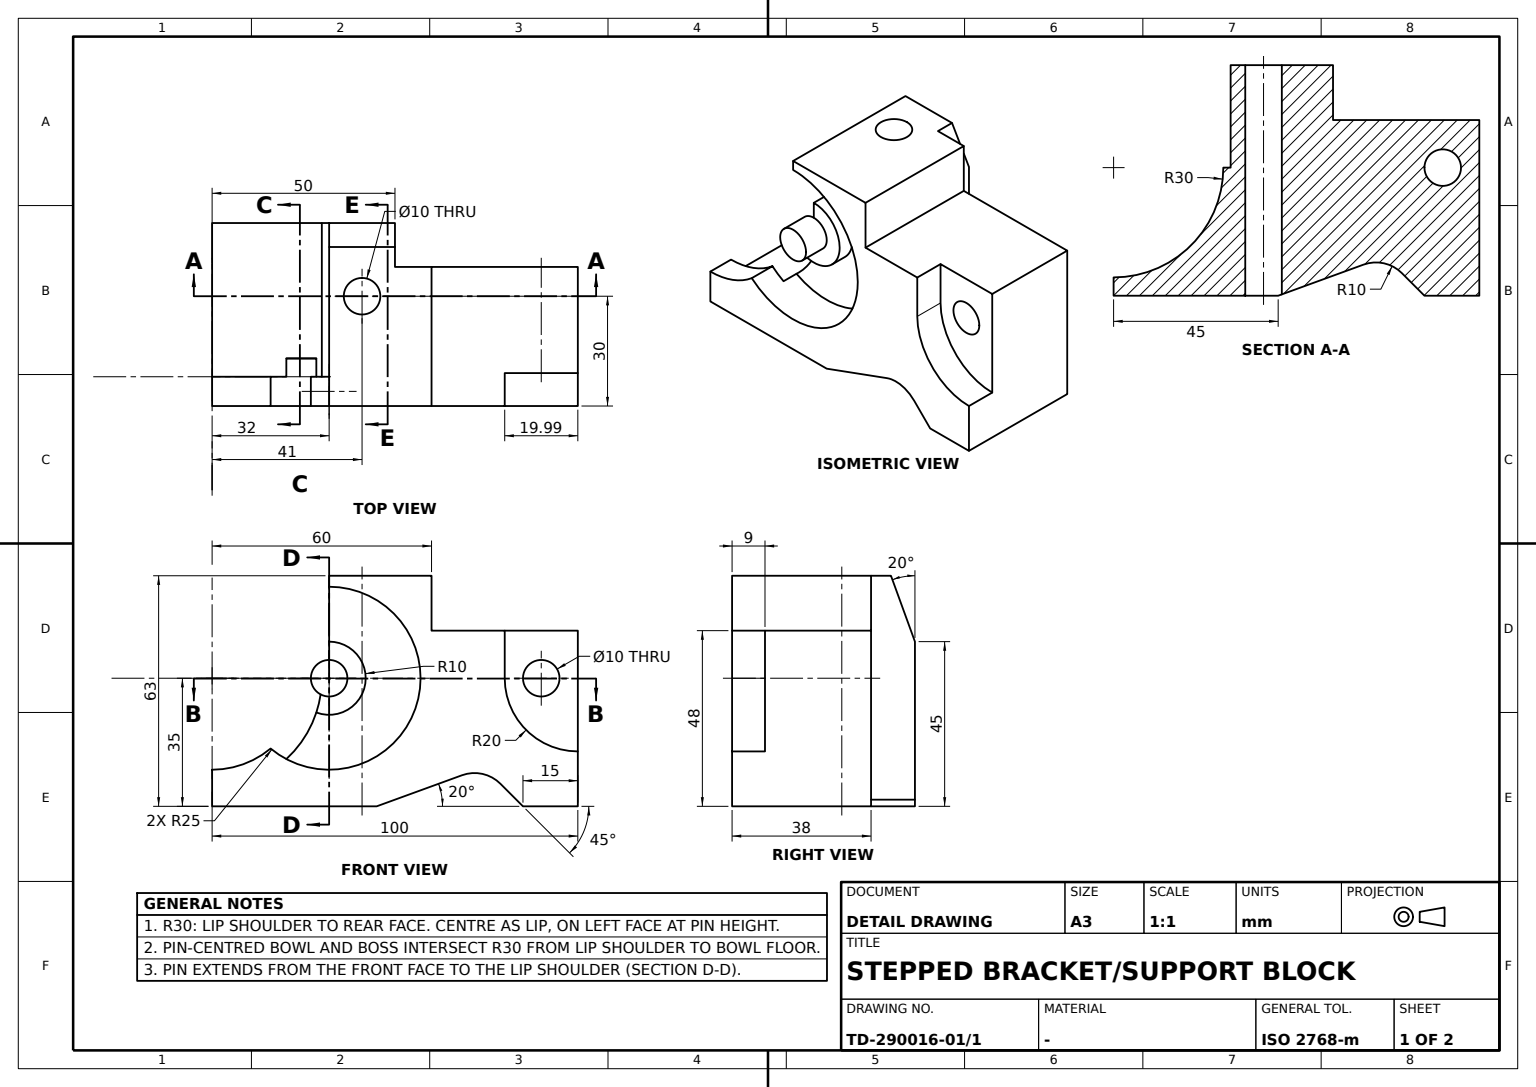
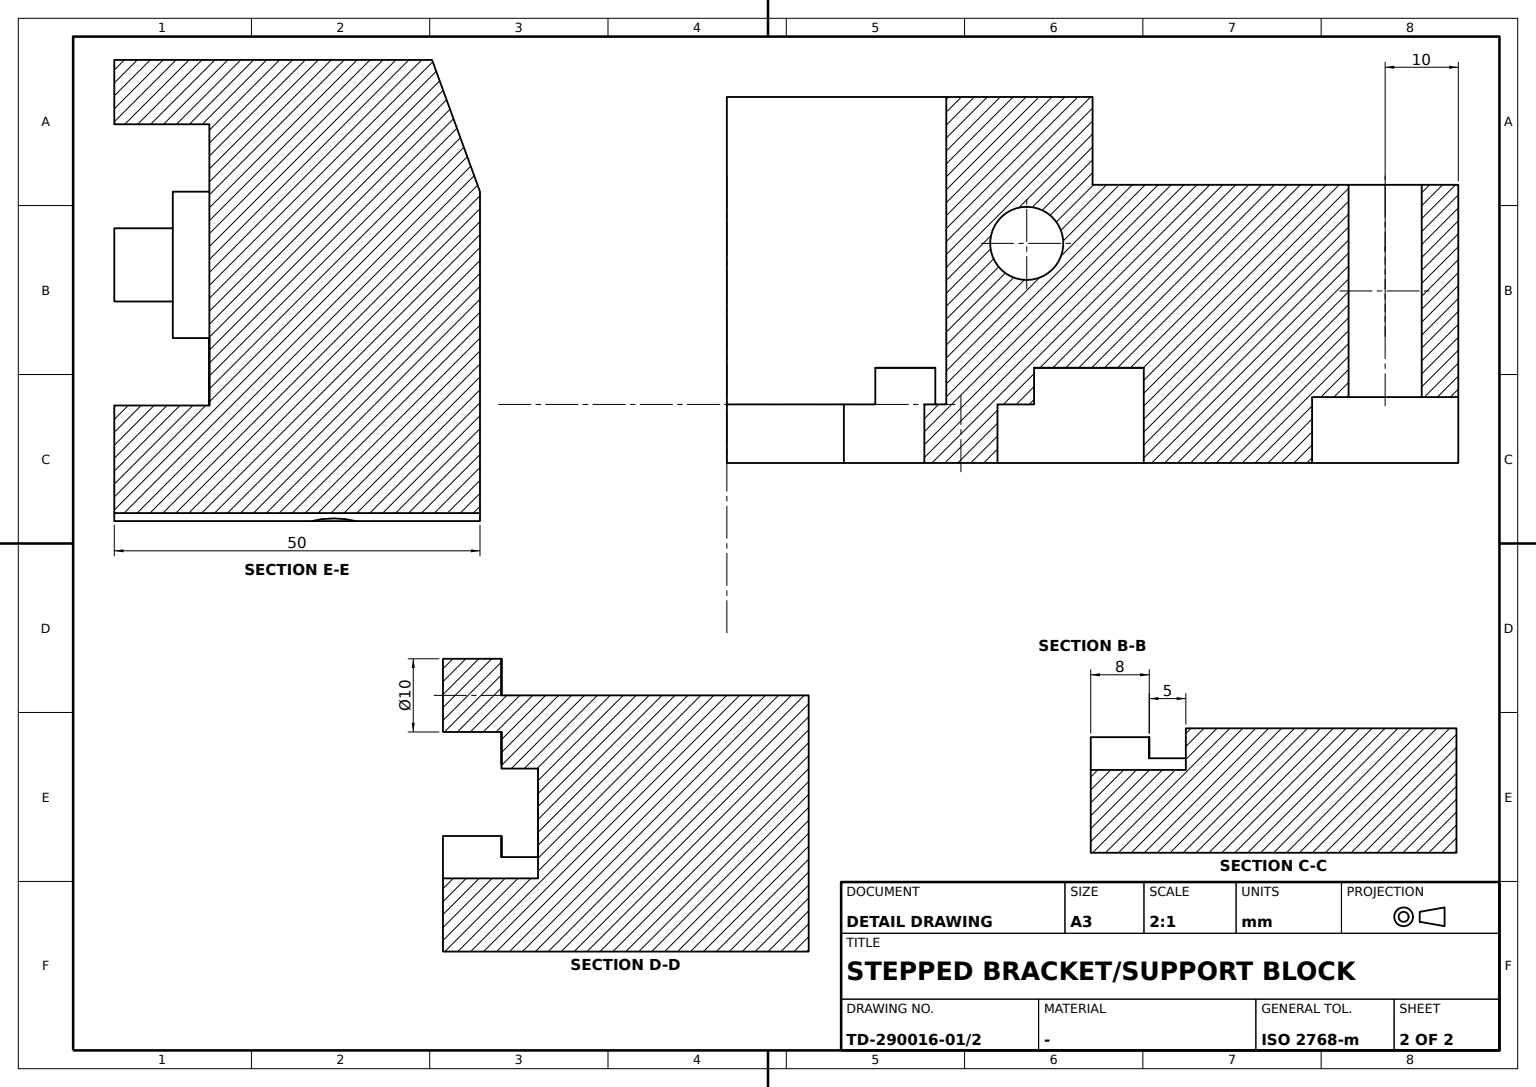
CATIA V5 part; units mm, degrees
sketch "Sketch1" plane through (0, 0, 0) normal (1, 0, 0) x (0, 1, 0)
  line L0 (0, 0) -> (100, 0)
  line L1 (0, 0) -> (0, 63)
  point P0 (0, 63)
  line L2 (0, 63) -> (100, 63)
  line L3 (100, 63) -> (100, 0)
  dimension "distance P0 origin" = 63
  dimension "length L2" = 100
  constraint horizontal L0 x-axis
  constraint horizontal L2 x-axis
  constraint vertical L1 y-axis
  constraint vertical L3 y-axis
extrude "Pad1" add sketch "Sketch1" along normal mid plane 50
sketch "Sketch2" plane through (25, 0, 0) normal (1, 0, 0) x (0, 1, 0)
  point P0 (80.0103, 63)
  point P1 (100.0103, 35)
  line L0 (0, 0) -> (100, 0) construction
  line L1 (100, 63) -> (0, 63) construction
  line L2 (80.0103, 63) -> (100.0103, 63)
  line L3 (100.0103, 63) -> (100.0103, 15)
  arc A0 (80.0103, 35) -> (100.0103, 15) centre (100.0103, 35) ccw
  line L4 (80.0103, 63) -> (80.0103, 35)
  point P2 (80.0103, 63)
  dimension "distance P1 L0" = 35
  dimension "distance P1 y axis" = 100.0103
  dimension "distance L3 y axis" = 100.0103
  dimension "radius A0" = 20
  constraint coincidence P0 L1
  constraint coincidence P0 L4
  constraint coincidence P2 L2
  constraint coincidence P0 P2
  constraint horizontal L2 x-axis
  constraint vertical L3 y-axis
  constraint vertical L4 y-axis
  constraint tangency L4 A0
extrude "Pocket1" cut sketch "Sketch2" against normal blind 9
sketch "Sketch3" plane through (0, 0, 63) normal (0, 0, 1) x (1, 0, 0)
  line L0 (-25, 100) -> (-13, 100)
  line L1 (-13, 100) -> (-13, 50)
  line L2 (-13, 50) -> (-25, 50)
  line L3 (-25, 50) -> (-25, 100)
  line L4 (-25, 100) -> (25, 100) construction
  line L5 (-25, 100) -> (-25, 0) construction
  dimension "length L3" = 50
  dimension "length L2" = 12
  constraint horizontal L0 x-axis
  constraint horizontal L2 x-axis
  constraint vertical L1 y-axis
  constraint vertical L3 y-axis
  constraint coincidence L0 L4
  constraint coincidence L3 L5
extrude "Pocket2" cut sketch "Sketch3" against normal through all
sketch "Sketch4" plane through (25, 0, 0) normal (1, 0, 0) x (0, 1, 0)
  line L0 (60, 63) -> (100, 63)
  line L1 (100, 63) -> (100, 48)
  line L2 (100, 48) -> (60, 48)
  line L3 (60, 48) -> (60, 63)
  line L4 (100, 63) -> (100, 15) construction
  line L5 (100, 63) -> (0, 63) construction
  dimension "length L0" = 40
  dimension "length L1" = 15
  constraint horizontal L0 x-axis
  constraint horizontal L2 x-axis
  constraint vertical L1 y-axis
  constraint vertical L3 y-axis
  constraint coincidence L1 L4
  constraint coincidence L0 L5
extrude "Pocket3" cut sketch "Sketch4" against normal through all
sketch "Sketch5" plane through (16, 0, 0) normal (1, 0, 0) x (0, 1, 0)
  circle A0 centre (90, 35) radius 5
  point P0 (90, 35)
  line L0 (100, 63) -> (100, 15) construction
  line L1 (0, 0) -> (100, 0) construction
  dimension "radius A0" = 5
  dimension "distance P0 L0" = 10
  dimension "distance P0 L1" = 35
extrude "Pocket4" cut sketch "Sketch5" against normal through all
sketch "Sketch6" plane through (25, 0, 0) normal (1, 0, 0) x (0, 1, 0)
  circle A0 centre (32, 35) radius 25
  point P0 (32, 35)
  line L0 (0, 0) -> (100, 0) construction
  line L1 (100, 63) -> (100, 15) construction
  dimension "radius A0" = 25
  dimension "distance P0 L0" = 35
  dimension "distance P0 L1" = 68
extrude "Pocket5" cut sketch "Sketch6" against normal blind 13
sketch "Sketch7" plane through (25, 0, 0) normal (1, 0, 0) x (0, 1, 0)
  circle A0 centre (0, 35) radius 30
  point P0 (0, 35)
  line L0 (0, 0) -> (100, 0) construction
  dimension "radius A0" = 30
  dimension "distance P0 L0" = 35
  constraint coincidence P0 y-axis
extrude "Pocket6" cut sketch "Sketch7" against normal through all
sketch "Sketch8" plane through (0, 0, 63) normal (0, 0, 1) x (1, 0, 0)
  line L0 (-33.3692, 32) -> (49.9529, 32)
  line L1 (-25, 50) -> (-13, 50) construction
  line L2 (-33.3692, 32) -> (-33.3692, -11.1214)
  line L3 (-33.3692, -11.1214) -> (49.9529, -11.1214)
  line L4 (49.9529, -11.1214) -> (49.9529, 32)
  dimension "distance L0 L1" = 18
  constraint horizontal L0 x-axis
  constraint horizontal L3 x-axis
  constraint vertical L2 y-axis
  constraint vertical L4 y-axis
extrude "Pocket7" cut sketch "Sketch8" against normal blind 28
sketch "Sketch9" plane through (12, 0, 0) normal (1, 0, 0) x (0, 1, 0)
  circle A0 centre (32, 35) radius 10
  circle A1 centre (32, 35) radius 25 construction
  dimension "radius A0" = 10
  constraint concentricity A0 A1
extrude "Pad2" add sketch "Sketch9" along normal blind 5
sketch "Sketch10" plane through (17, 0, 0) normal (1, 0, 0) x (0, 1, 0)
  arc A0 (0, 5) -> (30, 35) centre (0, 35) ccw
  line L0 (30, 35) -> (32, 35)
  line L1 (32, 63) -> (32, 35)
  line L2 (0, 5) -> (32, 63)
extrude "Pocket8" cut sketch "Sketch10" against normal blind 5
sketch "Sketch11" plane through (17, 0, 0) normal (1, 0, 0) x (0, 1, 0)
  circle A0 centre (32, 35) radius 5
  circle A1 centre (32, 35) radius 10 construction
  dimension "radius A0" = 5
  constraint concentricity A0 A1
extrude "Pad3" add sketch "Sketch11" along normal blind 8
sketch "Sketch12" plane through (0, 32, 0) normal (0, -1, 0) x (1, 0, 0)
  line L0 (-25, 45) -> (-18.4485, 63)
  point P0 (-25, 45)
  point P1 (-18.4485, 63)
  line L1 (-25, 63) -> (-25, 35) construction
  line L2 (25, 63) -> (-25, 63) construction
  line L3 (-18.4485, 63) -> (-25, 63)
  line L4 (-25, 63) -> (-25, 45)
  dimension "angle L0 L1" = 20
  dimension "distance P1 P0 y axis" = 18
  constraint coincidence P1 L2
  constraint coincidence P0 L1
  constraint horizontal L3 x-axis
  constraint vertical L4 y-axis
extrude "Pocket9" cut sketch "Sketch12" against normal up to next
sketch "Sketch13" plane through (0, 0, 63) normal (0, 0, 1) x (1, 0, 0)
  circle A0 centre (-5, 41) radius 5
  point P0 (-5, 41)
  line L0 (25, 100) -> (25, 0) construction
  line L1 (25, 32) -> (-25, 32) construction
  dimension "distance P0 L0" = 30
  dimension "distance P0 L1" = 9
  dimension "radius A0" = 5
extrude "Pocket10" cut sketch "Sketch13" against normal up to next
sketch "Sketch14" plane through (25, 0, 0) normal (1, 0, 0) x (0, 1, 0)
  line L0 (85, 0) -> (78.8309, 6.1691)
  point P0 (85, 0)
  line L1 (0, 0) -> (100, 0) construction
  line L2 (100, 0) -> (100, 63) construction
  line L3 (45, 0) -> (68.3397, 8.4949)
  point P1 (45, 0)
  line L4 (45, 0) -> (85, 0)
  point P2 (45, 0)
  arc A0 (68.3397, 8.4949) -> (78.8309, 6.1691) centre (71.7599, -0.902) cw
  dimension "angle L0 L1" = 45
  dimension "distance P0 L2" = 15
  dimension "angle L3 L1" = 20
  dimension "distance P1 P0" = 40
  dimension "radius A0" = 10
  constraint coincidence P0 x-axis
  constraint coincidence P1 x-axis
  constraint coincidence P1 P2
  constraint horizontal L4 x-axis
  constraint tangency A0 L3
  constraint tangency A0 L0
extrude "Pocket11" cut sketch "Sketch14" against normal up to next
sketch "Sketch15" plane through (25, 0, 0) normal (1, 0, 0) x (0, 1, 0)
  arc A0 (0, 10) -> (16, 15.7906) centre (0, 35) ccw
  point P0 (0, 35)
  line L0 (0, 0) -> (100, 0) construction
  arc A1 (16, 15.7906) -> (20.2969, 12.9084) centre (32, 35) ccw
  circle A2 centre (32, 35) radius 25 construction
  arc A3 (0, 5) -> (20.2969, 12.9084) centre (0, 35) ccw
  line L1 (0, 5) -> (0, 10)
  dimension "radius A0" = 25
  dimension "distance P0 L0" = 35
  constraint coincidence P0 y-axis
  constraint coincidence A1 A2
  constraint vertical L1 y-axis
extrude "Pad4" add sketch "Sketch15" against normal blind 8
